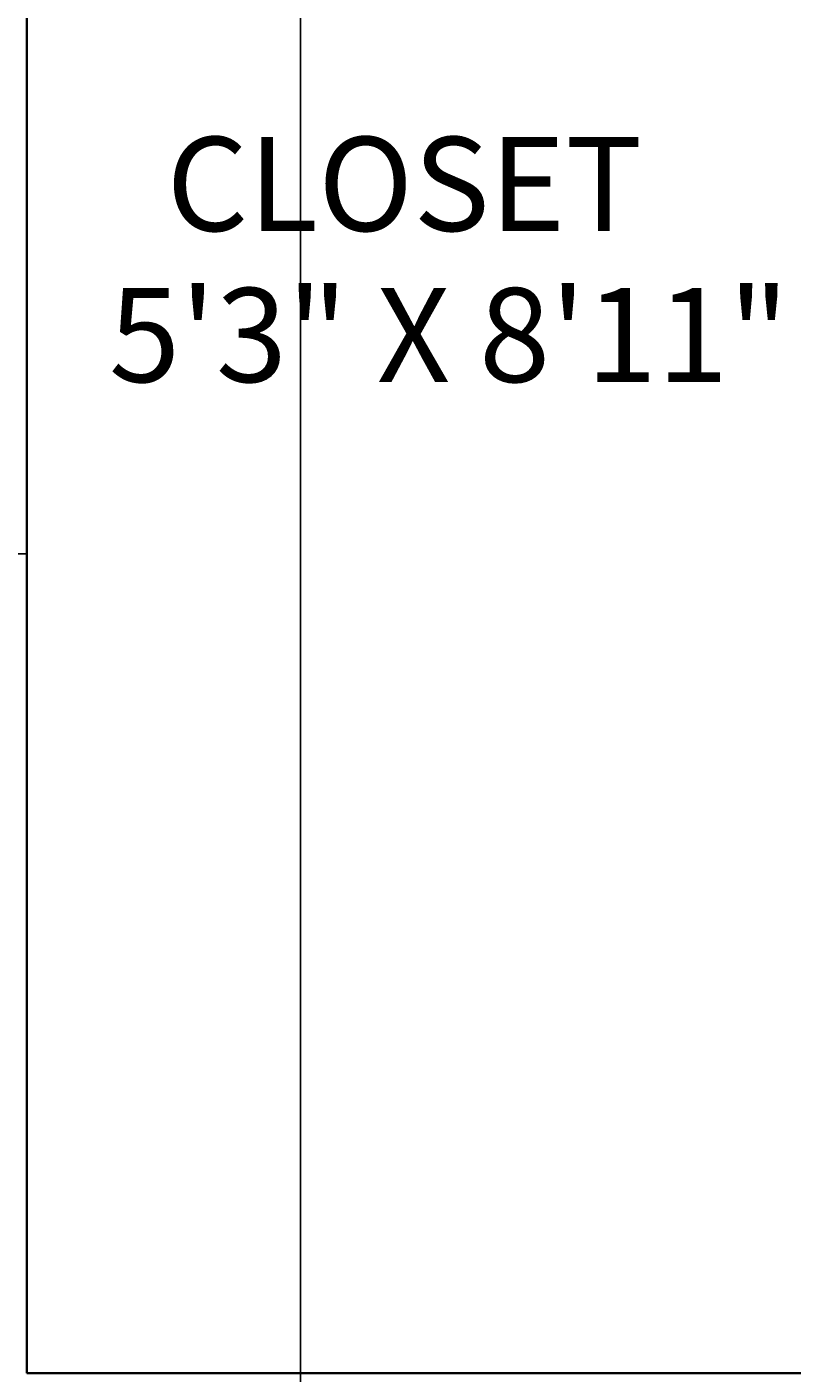
# Model space of a CAD drawing. Units: inches. Extents: x -61 to 1599, y -1316 to 257.
# Tile 63 of 204: x 166 to 205, y -282 to -213. Entities that reach past the tile are written whole.
import ezdxf

# ---------------------------------------------------------------- set-up
doc = ezdxf.new("R2010")
doc.units = ezdxf.units.IN
doc.header["$MEASUREMENT"] = 0
doc.linetypes.add('ACAD_ISO02W100', pattern=[15, 12, -3])
for name, color, linetype, lineweight in [('A-ANNO-DIMS', 2, 'Continuous', 18), ('A-AREA-IDEN', 1, 'Continuous', 18), ('A-WALL-JAMB', 4, 'ACAD_ISO02W100', 25), ('WALLS', 4, 'Continuous', 35)]:
    doc.layers.add(name, color=color, linetype=linetype, lineweight=lineweight)
doc.styles.get("Standard").update_dxf_attribs({"font": 'arial.ttf'})
doc.dimstyles.get("Standard").update_dxf_attribs({"dimtxt": 0.18, "dimasz": 0.18, "dimexe": 0.18, "dimexo": 0.0625, "dimgap": 0.09, "dimtad": 0, "dimtih": 1, "dimtoh": 1, "dimdec": 0, "dimzin": 0, "dimdsep": 46, "dimlunit": 3, "dimtxsty": 'Standard', "dimcen": 0.09, "dimadec": 0, "dimazin": 0, "dimtfac": 1, "dimtdec": 0, "dimtofl": 0, "dimtmove": 0, "dimatfit": 3, "dimfxl": 1, "dimtolj": 1, "dimtzin": 0, "dimarcsym": 0})

# ---------------------------------------------------------------- blocks, each defined once
blk = doc.blocks.new('*D687')
at = {"layer": 'A-ANNO-DIMS', "color": 0, "lineweight": -2, "transparency": 16777216}
for p, q in [((289.418, 181.677), (-61.077, 181.677)), ((-60.897, 181.497), (-60.897, -528.952)), ((-60.897, -1239.765), (-60.897, -529.316)), ((319.64, -1239.945), (-61.077, -1239.945))]:
    blk.add_line(p, q, dxfattribs=at)
at = {"layer": 'A-ANNO-DIMS', "color": 0, "transparency": 16777216}
for points in [[(-60.927, 181.497), (-60.867, 181.497), (-60.897, 181.677)], [(-60.927, -1239.765), (-60.867, -1239.765), (-60.897, -1239.945)]]:
    blk.add_solid(points, dxfattribs=at)
at = {"layer": 'DEFPOINTS', "color": 0, "transparency": 16777216}
for p in [(289.481, 181.677), (-60.897, -1239.945), (319.703, -1239.945)]:
    blk.add_point(p, dxfattribs=at)
at = {"layer": 'A-ANNO-DIMS', "color": 0, "transparency": 16777216, "insert": (-60.897, -529.134), "char_height": 0.18, "attachment_point": 5}
blk.add_mtext('\\A1;1421.6', dxfattribs=at)
blk = doc.blocks.new('*D699')
at = {"layer": 'A-ANNO-DIMS', "color": 0, "lineweight": -2, "transparency": 16777216}
for p, q in [((835.64, -167.169), (-61.077, -167.169)), ((-60.897, -167.349), (-60.897, -306.726)), ((-60.897, -446.466), (-60.897, -307.09)), ((841.64, -446.646), (-61.077, -446.646))]:
    blk.add_line(p, q, dxfattribs=at)
at = {"layer": 'A-ANNO-DIMS', "color": 0, "transparency": 16777216}
for points in [[(-60.927, -167.349), (-60.867, -167.349), (-60.897, -167.169)], [(-60.927, -446.466), (-60.867, -446.466), (-60.897, -446.646)]]:
    blk.add_solid(points, dxfattribs=at)
at = {"layer": 'DEFPOINTS', "color": 0, "transparency": 16777216}
for p in [(835.703, -167.169), (-60.897, -446.646), (841.703, -446.646)]:
    blk.add_point(p, dxfattribs=at)
at = {"layer": 'A-ANNO-DIMS', "color": 0, "transparency": 16777216, "insert": (-60.897, -306.908), "char_height": 0.18, "attachment_point": 5}
blk.add_mtext('\\A1;279.5', dxfattribs=at)
blk = doc.blocks.new('*D700')
at = {"layer": 'A-ANNO-DIMS', "color": 0, "lineweight": -2, "transparency": 16777216}
for p, q in [((14.703, -616.882), (14.703, 257.457)), ((14.883, 257.277), (96.772, 257.277)), ((179.572, 257.277), (97.683, 257.277)), ((179.752, -616.882), (179.752, 257.457))]:
    blk.add_line(p, q, dxfattribs=at)
at = {"layer": 'A-ANNO-DIMS', "color": 0, "transparency": 16777216}
for points in [[(14.883, 257.307), (14.883, 257.247), (14.703, 257.277)], [(179.572, 257.307), (179.572, 257.247), (179.752, 257.277)]]:
    blk.add_solid(points, dxfattribs=at)
at = {"layer": 'DEFPOINTS', "color": 0, "transparency": 16777216}
for p in [(179.752, 257.277), (14.703, -616.945), (179.752, -616.945)]:
    blk.add_point(p, dxfattribs=at)
at = {"layer": 'A-ANNO-DIMS', "color": 0, "transparency": 16777216, "insert": (97.227, 257.277), "char_height": 0.18, "attachment_point": 5}
blk.add_mtext('\\A1;165.05', dxfattribs=at)

msp = doc.modelspace()

# ---------------------------------------------------------------- linework, layer by layer
at = {"layer": 'A-WALL-JAMB'}
msp.add_line((165.7028, -240.2369), (159.7028, -240.2369), dxfattribs=at)
at = {"layer": 'WALLS'}
for q in [(165.7028, -175.3229), (228.7028, -282.3229)]:
    msp.add_line((165.7028, -282.3229), q, dxfattribs=at)

# ---------------------------------------------------------------- texts
at = {"layer": 'A-AREA-IDEN'}
for s, height, p in [('  CLOSET', 4.8321, (169.9149, -223.6457)), ('5\'3" X 8\'11"', 4.832098, (169.9149, -231.408))]:
    msp.add_text(s, height=height, dxfattribs=at).set_placement(p)

# ---------------------------------------------------------------- dimensions: what is measured, and where the dimension line sits
at = {"layer": 'A-ANNO-DIMS'}
dim = msp.add_linear_dim(base=(179.7521, 257.2771), p1=(14.7028, -616.9446), p2=(179.7521, -616.9446), dimstyle='Standard', override={"dimdec": 2, "dimlfac": 1, "dimrnd": 0, "dimzin": 0, "dimdsep": 46, "dimlunit": 2}, dxfattribs=at)
dim.commit()
dim.dimension.update_dxf_attribs({"geometry": '*D700', "text_midpoint": (97.2274, 257.2771)})
for base, p1, p2, picture, middle in [((-60.8972, -1239.9446), (289.4807, 181.6771), (319.7028, -1239.9446), '*D687', (-60.8972, -529.1337)), ((-60.8972, -446.6462), (835.7028, -167.169), (841.7028, -446.6462), '*D699', (-60.8972, -306.9076))]:
    dim = msp.add_linear_dim(base=base, p1=p1, p2=p2, angle=90, dimstyle='Standard', override={"dimdec": 1, "dimlfac": 1, "dimrnd": 0, "dimzin": 0, "dimdsep": 46, "dimlunit": 2}, dxfattribs=at)
    dim.commit()
    dim.dimension.update_dxf_attribs({"geometry": picture, "text_midpoint": middle})

doc.saveas('drawing.dxf')
